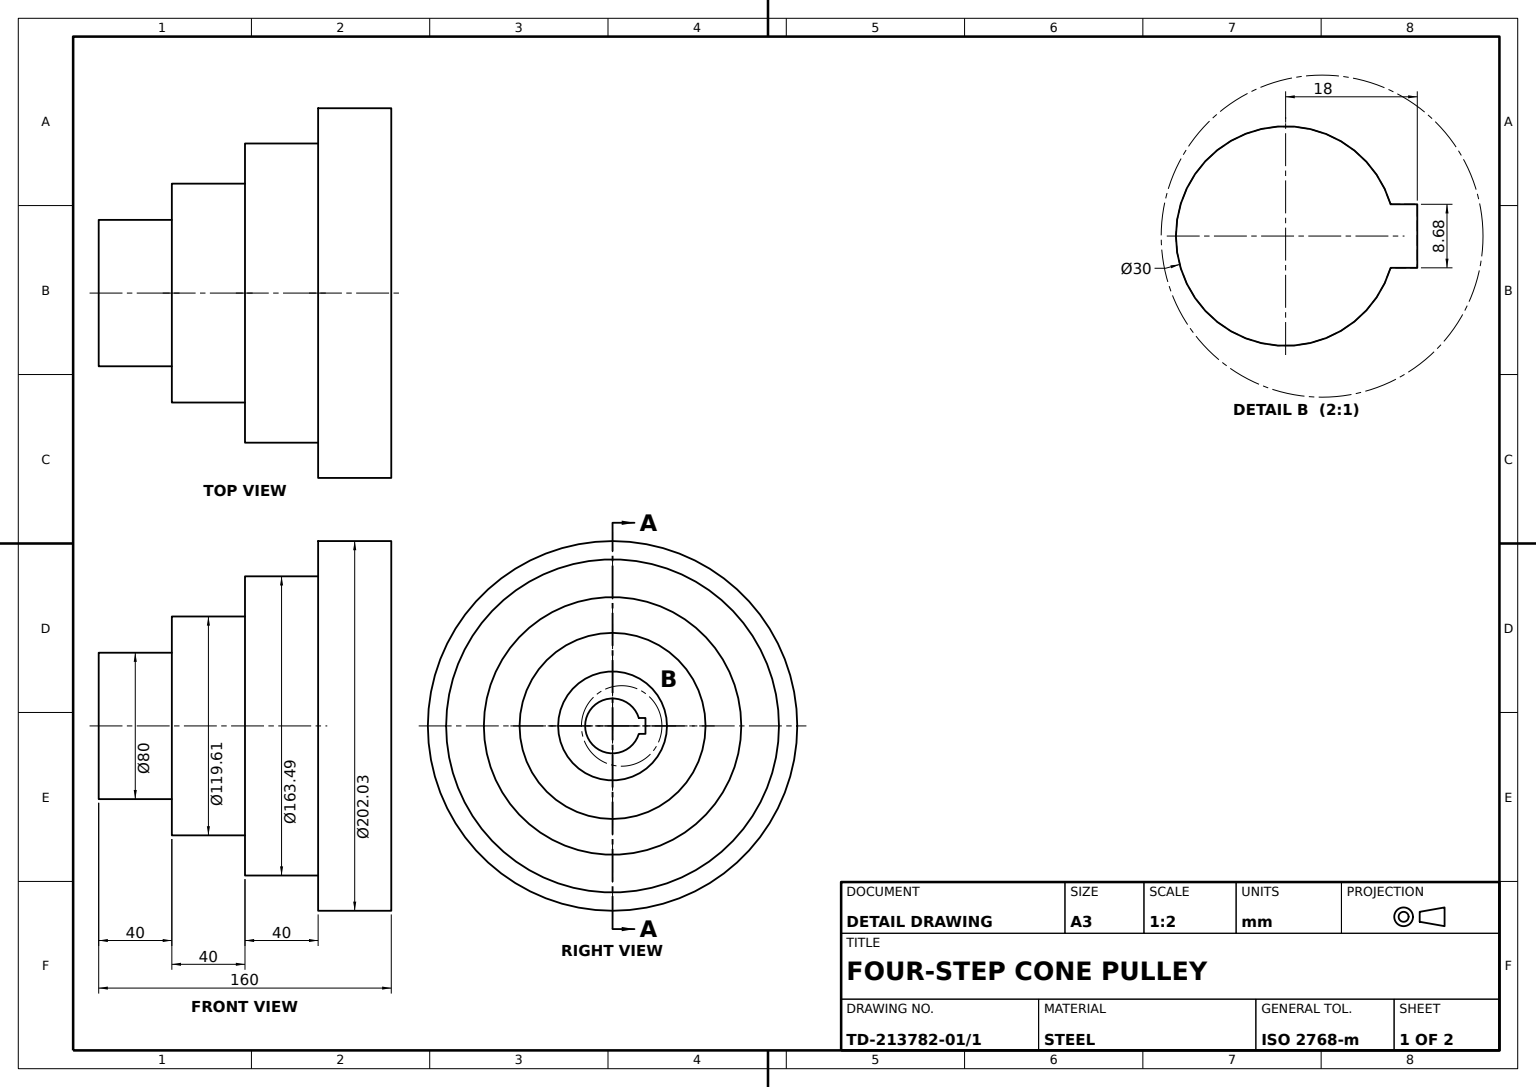
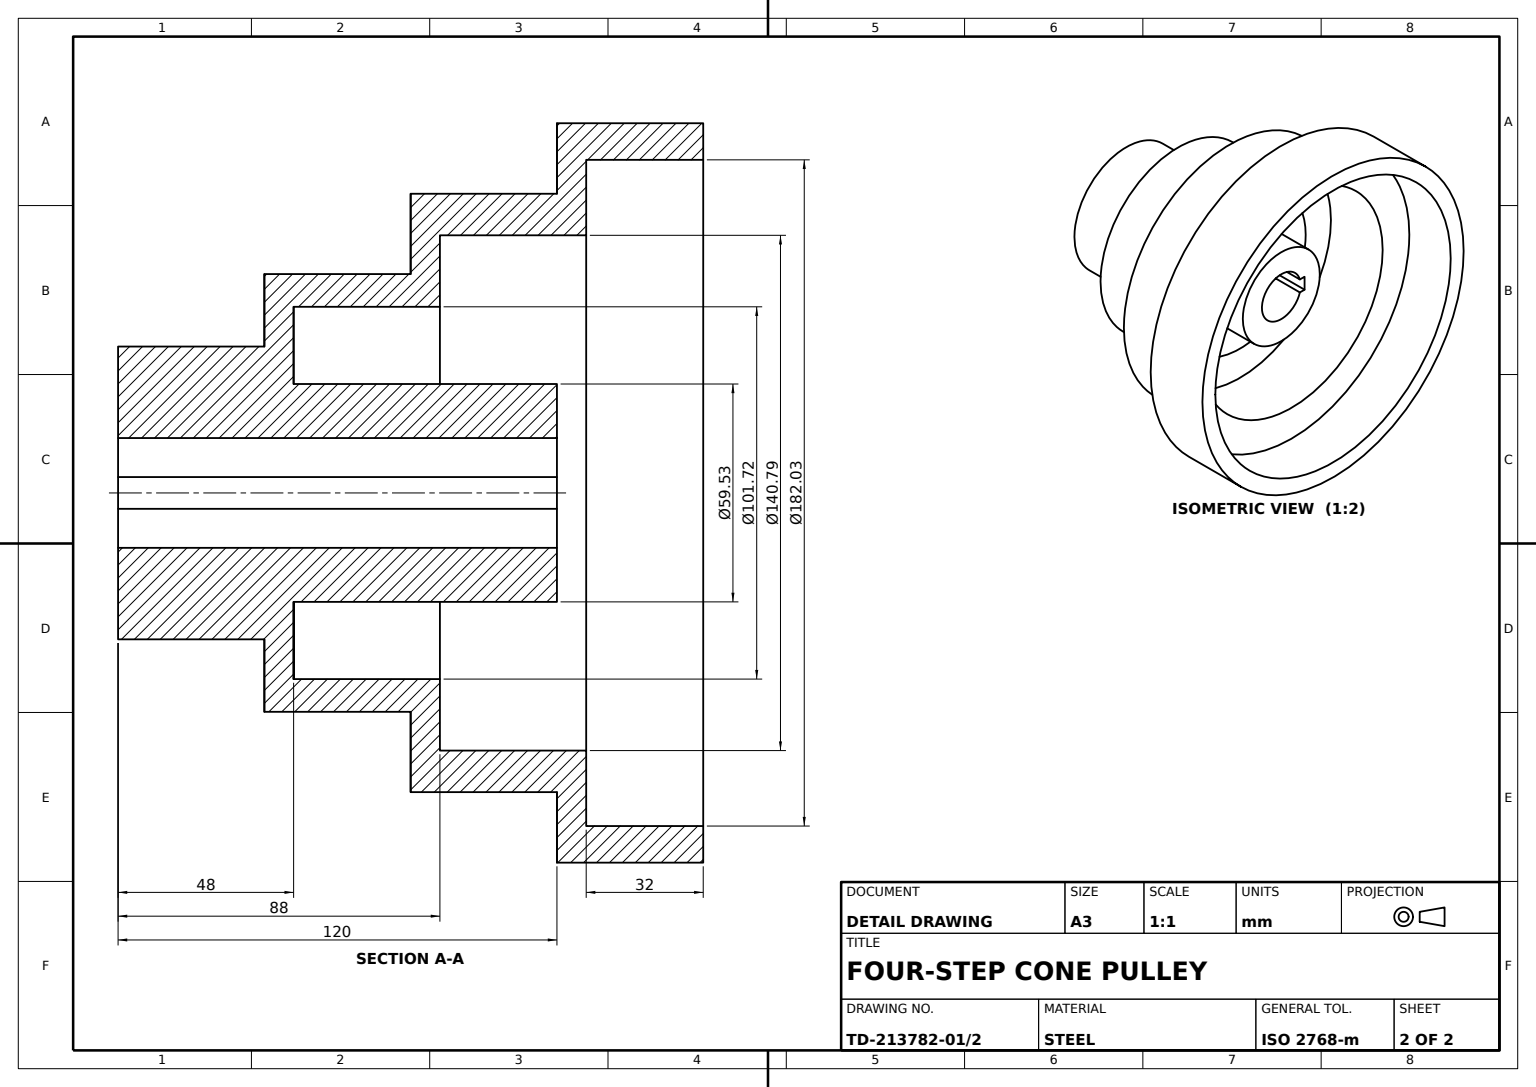
SolidWorks part; units mm, degrees
material "Plain Carbon Steel"
ref_plane "Front Plane" through (0, 0, 0) normal (0, 0, 1) x (1, 0, 0)
ref_plane "Top Plane" through (0, 0, 0) normal (0, 1, 0) x (1, 0, 0)
ref_plane "Right Plane" through (0, 0, 0) normal (1, 0, 0) x (0, 0, -1)
sketch "Stepped Pulley Profile" plane through (0, 0, 0) normal (0, 0, 1) x (1, 0, 0)
  line L0 (151.6898, 0) -> (-160.8831, 0) construction
  line L1 (0, -157.8187) -> (0, 189.9953) construction
  line L2 (-55.07, 15) -> (-55.07, 40)
  line L3 (-55.07, 40) -> (-15.07, 40)
  line L4 (-15.07, 40) -> (-15.07, 59.8026)
  line L5 (-15.07, 59.8026) -> (24.93, 59.8026)
  line L6 (24.93, 59.8026) -> (24.93, 81.7461)
  line L7 (24.93, 81.7461) -> (64.93, 81.7461)
  line L8 (64.93, 81.7461) -> (64.93, 101.0135)
  line L9 (64.93, 101.0135) -> (104.93, 101.0135)
  line L10 (104.93, 101.0135) -> (104.93, 91.0135)
  line L11 (104.93, 91.0135) -> (72.93, 91.0135)
  line L12 (72.93, 91.0135) -> (72.93, 70.3938)
  line L13 (72.93, 70.3938) -> (32.93, 70.3938)
  line L14 (32.93, 70.3938) -> (32.93, 50.8588)
  line L15 (32.93, 50.8588) -> (-7.07, 50.8588)
  line L16 (-7.07, 50.8588) -> (-7.07, 29.7651)
  line L17 (-7.07, 29.7651) -> (64.93, 29.7651)
  line L18 (64.93, 29.7651) -> (64.93, 15)
  line L19 (64.93, 15) -> (-55.07, 15)
  dimension "D1" = 24.93
  dimension "D2" = 32.93
  dimension "D3" = 64.93
  dimension "D4" = 15
  dimension "D5" = 29.7651
  dimension "D6" = 40
  dimension "D7" = 50.8588
  dimension "D8" = 59.8026
  dimension "D9" = 70.3938
  dimension "D10" = 81.7461
  dimension "D11" = 91.0135
  dimension "D12" = 101.0135
revolve "Stepped Pulley Body" add sketch "Stepped Pulley Profile" angle 360 about L0
sketch "Bore and Keyway Profile" plane through (0, 0, 0) normal (1, 0, 0) x (0, 0, -1)
  line L1 (3, 4.3401) -> (18, 4.3401)
  line L2 (3, 4.3401) -> (3, -4.3401)
  line L3 (3, -4.3401) -> (18, -4.3401)
  line L4 (18, 4.3401) -> (18, -4.3401)
  point P5 (3, 0)
  dimension "D1" = 15
  dimension "D2" = 8.6802
  dimension "D3" = 18
extrude "Shaft Bore with Keyway" cut sketch "Bore and Keyway Profile" against normal mid plane 220
